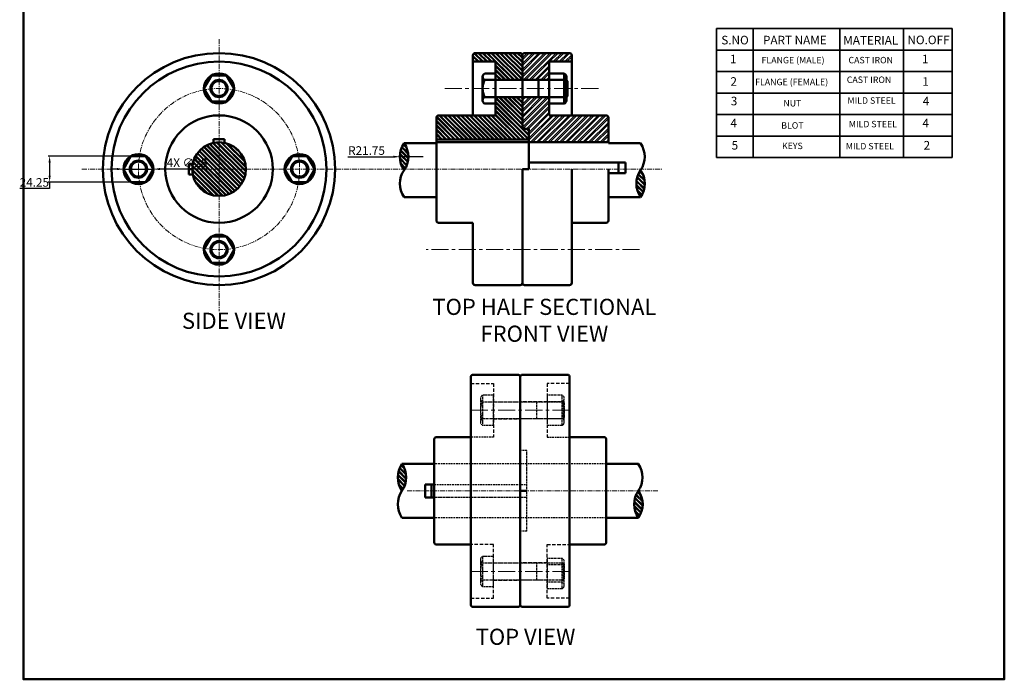
# Model space of a CAD drawing. Units: millimetres. Extents: x 36 to 952, y -590 to 448.
# Tile 1 of 2: x 36 to 952, y -590 to 24. Entities that reach past the tile are written whole.
import ezdxf

# ---------------------------------------------------------------- set-up
doc = ezdxf.new("R2010")
doc.units = ezdxf.units.MM
doc.header["$LTSCALE"] = 0.5
doc.linetypes.add('CENTER', pattern=[50.8, 31.75, -6.35, 6.35, -6.35])
doc.linetypes.add('HIDDEN', pattern=[9.525, 6.35, -3.175])
for name, color, linetype, lineweight in [('M-CNTR', 1, 'CENTER', 18), ('M-DIMS', 2, 'Continuous', 25), ('M-HATC', 8, 'Continuous', 18), ('M-HIDN', 4, 'HIDDEN', 25), ('M-OUTL', 7, 'Continuous', 50), ('M-TEXT', 7, 'Continuous', 25), ('M-TTLB', 7, 'Continuous', 35)]:
    doc.layers.add(name, color=color, linetype=linetype, lineweight=lineweight)
doc.styles.get("Standard").update_dxf_attribs({"font": 'arial.ttf'})
doc.dimstyles.new('ISO-25', dxfattribs={"dimtxt": 8, "dimasz": 6, "dimexe": 1.25, "dimexo": 0.625, "dimtad": 1, "dimtoh": 1, "dimtxsty": 'Standard', "dimcen": 2.5, "dimadec": 0, "dimazin": 0, "dimtfac": 1, "dimtmove": 0, "dimatfit": 3, "dimfxl": 1, "dimarcsym": 0})
pattern_1 = [(135, (903.4658, -449.5868), (-2.020558, -2.020558), []), (135, (903.4658, -448.2397), (-2.020558, -2.020558), [])]

# ---------------------------------------------------------------- blocks, each defined once
blk = doc.blocks.new('NUT-HEX')
at = {"ltscale": 0.3}
blk.add_lwpolyline([(28, 14), (21, 26.12), (7, 26.12), (0, 14), (7, 1.88), (21, 1.88)], close=True, dxfattribs=at)
blk.add_circle((14, 14), 14, dxfattribs=at)
blk = doc.blocks.new('*D27')
at = {"layer": 'Defpoints', "color": 0, "ltscale": 0.5, "transparency": 16777216}
for p in [(139.37, -102.71), (63.75, -126.96), (139.37, -126.96)]:
    blk.add_point(p, dxfattribs=at)
at = {"layer": 'M-DIMS', "color": 0, "lineweight": -2, "ltscale": 0.5, "transparency": 16777216}
for p, q in [((138.74, -102.71), (62.5, -102.71)), ((63.75, -108.71), (63.75, -120.96)), ((138.74, -126.96), (62.5, -126.96)), ((63.75, -126.96), (63.75, -132.96)), ((63.75, -132.96), (35.94, -132.96))]:
    blk.add_line(p, q, dxfattribs=at)
at = {"layer": 'M-DIMS', "color": 0, "ltscale": 0.5, "transparency": 16777216}
for points in [[(62.75, -108.71), (64.75, -108.71), (63.75, -102.71)], [(62.75, -120.96), (64.75, -120.96), (63.75, -126.96)]]:
    blk.add_solid(points, dxfattribs=at)
at = {"layer": 'M-DIMS', "color": 0, "ltscale": 0.5, "transparency": 16777216, "insert": (49.53, -128.25), "char_height": 8, "attachment_point": 5}
blk.add_mtext('24.25', dxfattribs=at)
blk = doc.blocks.new('*D30')
at = {"layer": 'Defpoints', "color": 0, "ltscale": 0.5, "transparency": 16777216}
for p in [(132.37, -114.83), (160.37, -114.83)]:
    blk.add_point(p, dxfattribs=at)
at = {"layer": 'M-DIMS', "color": 0, "lineweight": -2, "ltscale": 0.5, "transparency": 16777216}
for p, q in [((126.37, -114.83), (120.37, -114.83)), ((132.37, -114.83), (160.37, -114.83)), ((172.37, -114.83), (166.37, -114.83)), ((210.26, -114.83), (172.37, -114.83))]:
    blk.add_line(p, q, dxfattribs=at)
at = {"layer": 'M-DIMS', "color": 0, "ltscale": 0.5, "transparency": 16777216}
for points in [[(126.37, -113.83), (126.37, -115.83), (132.37, -114.83)], [(166.37, -113.83), (166.37, -115.83), (160.37, -114.83)]]:
    blk.add_solid(points, dxfattribs=at)
at = {"layer": 'M-DIMS', "color": 0, "ltscale": 0.5, "transparency": 16777216, "insert": (191.62, -109.9), "char_height": 8, "attachment_point": 5}
blk.add_mtext('4X ∅28', dxfattribs=at)
blk = doc.blocks.new('*D31')
at = {"layer": 'Defpoints', "color": 0, "ltscale": 0.5, "transparency": 16777216}
for p in [(389.66, -103.33), (411.41, -103.33)]:
    blk.add_point(p, dxfattribs=at)
at = {"layer": 'M-DIMS', "color": 0, "lineweight": -2, "ltscale": 0.5, "transparency": 16777216}
for p, q in [((341.28, -103.33), (376.61, -103.33)), ((376.61, -103.33), (383.66, -103.33)), ((411.41, -103.33), (389.66, -103.33))]:
    blk.add_line(p, q, dxfattribs=at)
at = {"layer": 'M-DIMS', "color": 0, "ltscale": 0.5, "transparency": 16777216}
blk.add_solid([(383.66, -102.33), (383.66, -104.33), (389.66, -103.33)], dxfattribs=at)
at = {"layer": 'M-DIMS', "color": 0, "ltscale": 0.5, "transparency": 16777216, "insert": (358.63, -98.62), "char_height": 8, "attachment_point": 5}
blk.add_mtext('R21.75', dxfattribs=at)

msp = doc.modelspace()

# ---------------------------------------------------------------- hatches: boundary and pattern name
at = {"layer": 'M-HATC', "ltscale": 0.3}
h = msp.add_hatch(dxfattribs=at)
h.set_pattern_fill('ANSI32', color=256, scale=0.3, angle=90)
h.set_pattern_definition([(135, (649.1825, -488.8874), (-2.020558, -2.020558), []), (135, (649.1825, -487.5403), (-2.020558, -2.020558), [])])
h.paths.add_polyline_path([(459.614, -6.832, 0.4142136), (457.614, -8.832), (457.614, -14.832), (478.614, -14.832), (478.614, -31.832), (503.614, -31.832), (503.614, -8.832, 0.4142136), (501.614, -6.832)])
h = msp.add_hatch(dxfattribs=at)
h.set_pattern_fill('ANSI32', color=256, scale=0.4)
h.set_pattern_definition([(45, (47.152, -333.0392), (-2.694077, 2.694077), []), (45, (48.948, -333.0392), (-2.694077, 2.694077), [])])
h.paths.add_polyline_path([(528.614, -14.832), (549.614, -14.832), (549.614, -8.832, 0.4142136), (547.614, -6.832), (505.614, -6.832, 0.4142136), (503.614, -8.832), (503.614, -31.832), (528.614, -31.832)])
h.paths.add_polyline_path([(503.614, -77.332), (509.614, -77.332), (509.614, -89.832), (583.614, -89.832), (583.614, -66.832, 0.4142136), (581.614, -64.832), (528.614, -64.832), (528.614, -47.832), (503.614, -47.832)])
h = msp.add_hatch(dxfattribs=at)
h.set_pattern_fill('ANSI32', color=256, scale=0.3, angle=90)
h.set_pattern_definition(pattern_1)
h.paths.add_polyline_path([(478.614, -64.832), (425.614, -64.832, 0.4142136), (423.614, -66.832), (423.614, -87.332), (509.614, -87.332), (509.614, -77.332), (503.614, -77.332), (503.614, -47.832), (478.614, -47.832)])
h = msp.add_hatch(dxfattribs=at)
h.set_pattern_fill('ANSI32', color=256, scale=0.3, angle=90)
h.set_pattern_definition([(135, (1009.3846, -92.6427), (-2.020558, -2.020558), []), (135, (1009.3846, -91.2956), (-2.020558, -2.020558), [])])
h.paths.add_polyline_path([(196.366, -114.832), (246.366, -114.832, 1)])
h.paths.add_polyline_path([(246.366, -114.832), (196.366, -114.832, 1)])
h = msp.add_hatch(dxfattribs=at)
h.set_pattern_fill('ANSI32', color=256, scale=0.3, angle=90)
h.set_pattern_definition(pattern_1)
h.paths.add_polyline_path([(393.614, -115.832, 0.31606), (393.614, -90.832, 0.31606)])
h = msp.add_hatch(dxfattribs=at)
h.set_pattern_fill('ANSI32', color=256, scale=0.3, angle=90)
h.set_pattern_definition([(135, (1123.4658, -474.5868), (-2.020558, -2.020558), []), (135, (1123.4658, -473.2397), (-2.020558, -2.020558), [])])
h.paths.add_polyline_path([(613.614, -140.832, 0.31606), (613.614, -115.832, 0.31606)])
h = msp.add_hatch(dxfattribs=at)
h.set_pattern_fill('ANSI32', color=256, scale=0.3, angle=90)
h.set_pattern_definition([(135, (901.4658, -748.1027), (-2.020558, -2.020558), []), (135, (901.4658, -746.7557), (-2.020558, -2.020558), [])])
h.paths.add_polyline_path([(391.614, -414.348, 0.31606), (391.614, -389.348, 0.31606)])
h = msp.add_hatch(dxfattribs=at)
h.set_pattern_fill('ANSI32', color=256, scale=0.3, angle=90)
h.set_pattern_definition([(135, (1121.4658, -773.1027), (-2.020558, -2.020558), []), (135, (1121.4658, -771.7557), (-2.020558, -2.020558), [])])
h.paths.add_polyline_path([(611.614, -439.348, 0.31606), (611.614, -414.348, 0.31606)])

# ---------------------------------------------------------------- linework, layer by layer
at = {"layer": 'M-CNTR', "ltscale": 0.3}
for p, q in [((221.366, 6.13), (221.366, -247.228)), ((93.755, -114.832), (633.407, -114.832)), ((396.436, -414.348), (629.872, -414.348))]:
    msp.add_line(p, q, dxfattribs=at)
at = {"layer": 'M-CNTR'}
for p, q in [((574.352, -39.832), (431.256, -39.832)), ((612.663, -189.832), (414.062, -189.832)), ((455.614, -339.348), (501.614, -339.348)), ((547.614, -339.348), (501.614, -339.348)), ((455.614, -489.348), (501.614, -489.348)), ((547.614, -489.348), (501.614, -489.348))]:
    msp.add_line(p, q, dxfattribs=at)
at = {"layer": 'M-CNTR', "ltscale": 0.3}
msp.add_circle((221.366, -114.832), 75, dxfattribs=at)
at = {"layer": 'M-HIDN'}
for p, q in [((455.614, -314.348), (476.614, -314.348)), ((476.614, -314.348), (476.614, -364.348)), ((547.614, -314.348), (526.614, -314.348)), ((526.614, -314.348), (526.614, -364.348)), ((476.614, -331.348), (501.614, -331.348)), ((526.614, -331.348), (501.614, -331.348)), ((476.614, -347.348), (501.614, -347.348)), ((526.614, -347.348), (501.614, -347.348)), ((476.614, -464.348), (455.614, -464.348)), ((476.614, -514.348), (476.614, -464.348)), ((526.614, -514.348), (526.614, -464.348)), ((526.614, -464.348), (547.614, -464.348)), ((476.614, -481.348), (501.614, -481.348)), ((526.614, -481.348), (501.614, -481.348)), ((476.614, -497.348), (501.614, -497.348)), ((526.614, -497.348), (501.614, -497.348)), ((455.614, -514.348), (476.614, -514.348)), ((547.614, -514.348), (526.614, -514.348))]:
    msp.add_line(p, q, dxfattribs=at)
at = {"layer": 'M-HIDN', "ltscale": 0.3}
for p, q in [((464.614, -328.348), (464.614, -347.348)), ((476.614, -325.348), (466.614, -325.348)), ((466.614, -325.348), (466.614, -353.348)), ((476.614, -331.348), (476.614, -325.348)), ((540.614, -325.348), (526.614, -325.348)), ((526.614, -325.348), (526.614, -353.348)), ((540.614, -353.348), (540.614, -325.348)), ((542.614, -350.348), (542.614, -328.348)), ((464.614, -331.348), (541.614, -331.348)), ((476.614, -347.348), (476.614, -331.348)), ((516.614, -331.348), (516.614, -347.348)), ((540.614, -331.348), (526.614, -331.348)), ((542.614, -332.348), (541.614, -331.348)), ((541.614, -331.348), (541.614, -347.348)), ((542.614, -332.348), (542.614, -346.348)), ((541.614, -347.348), (464.614, -347.348)), ((464.614, -347.348), (464.614, -350.348)), ((476.614, -353.348), (476.614, -347.348)), ((540.614, -347.348), (526.614, -347.348)), ((542.614, -346.348), (541.614, -347.348)), ((466.614, -353.348), (476.614, -353.348)), ((526.614, -353.348), (540.614, -353.348)), ((507.614, -420.598), (421.614, -420.598)), ((476.614, -475.348), (466.614, -475.348)), ((466.614, -475.348), (466.614, -503.348)), ((476.614, -481.348), (476.614, -475.348)), ((464.614, -478.348), (464.614, -497.348)), ((464.614, -481.348), (541.614, -481.348)), ((476.614, -497.348), (476.614, -481.348)), ((516.614, -481.348), (516.614, -497.348)), ((540.614, -477.348), (526.614, -477.348)), ((526.614, -477.348), (526.614, -505.348)), ((540.614, -483.348), (526.614, -483.348)), ((540.614, -505.348), (540.614, -477.348)), ((542.614, -482.348), (541.614, -481.348)), ((541.614, -481.348), (541.614, -497.348)), ((542.614, -502.348), (542.614, -480.348)), ((542.614, -482.348), (542.614, -496.348)), ((541.614, -497.348), (464.614, -497.348)), ((464.614, -497.348), (464.614, -500.348)), ((466.614, -503.348), (476.614, -503.348)), ((476.614, -503.348), (476.614, -497.348)), ((540.614, -499.348), (526.614, -499.348)), ((542.614, -496.348), (541.614, -497.348)), ((526.614, -505.348), (540.614, -505.348))]:
    msp.add_line(p, q, dxfattribs=at)
at = {"layer": 'M-HIDN', "ltscale": 0.5}
for p, q in [((476.614, -364.348), (455.614, -364.348)), ((526.614, -364.348), (547.614, -364.348)), ((507.614, -376.848), (501.614, -376.848)), ((581.614, -389.348), (421.614, -389.348)), ((421.614, -408.598), (507.614, -408.598)), ((581.614, -439.348), (421.614, -439.348)), ((507.614, -451.848), (501.614, -451.848))]:
    msp.add_line(p, q, dxfattribs=at)
at = {"layer": 'M-HIDN', "ltscale": 0.3}
msp.add_lwpolyline([(507.614, -451.848), (507.614, -414.348), (507.614, -376.848)], dxfattribs=at)
for centre, radius, start, end in [((467.864, -328.348), 3.25, 112.619865, 247.380135), ((539.364, -328.348), 3.25, 292.619865, 67.380135), ((481.614, -339.348), 17, 151.927513, 208.072487), ((525.614, -339.348), 17, 331.927513, 28.072487), ((467.864, -350.348), 3.25, 112.619865, 247.380135), ((539.364, -350.348), 3.25, 292.619865, 67.380135), ((467.864, -478.348), 3.25, 112.619865, 247.380135), ((481.614, -489.348), 17, 151.927513, 208.072487), ((539.364, -480.348), 3.25, 292.619865, 67.380135), ((525.614, -491.348), 17, 331.927513, 28.072487), ((467.864, -500.348), 3.25, 112.619865, 247.380135), ((539.364, -502.348), 3.25, 292.619865, 67.380135)]:
    msp.add_arc(centre, radius, start, end, dxfattribs=at)
at = {"layer": 'M-OUTL'}
for p, q in [((457.614, -8.832), (457.614, -64.832)), ((459.614, -6.832), (501.614, -6.832)), ((503.614, -8.832), (503.614, -77.332)), ((503.614, -8.832), (503.614, -77.332)), ((505.614, -6.832), (547.614, -6.832)), ((549.614, -8.832), (549.614, -64.832)), ((457.614, -14.832), (478.614, -14.832)), ((478.614, -14.832), (478.614, -64.832)), ((549.614, -14.832), (528.614, -14.832)), ((528.614, -14.832), (528.614, -64.832)), ((478.614, -31.832), (503.614, -31.832)), ((528.614, -31.832), (503.614, -31.832)), ((478.614, -47.832), (503.614, -47.832)), ((528.614, -47.832), (503.614, -47.832)), ((423.614, -66.832), (423.614, -114.832)), ((478.614, -64.832), (425.614, -64.832)), ((528.614, -64.832), (581.614, -64.832)), ((583.614, -66.832), (583.614, -90.832)), ((503.614, -77.332), (508.614, -77.332)), ((509.614, -87.332), (423.614, -87.332)), ((509.614, -89.832), (423.614, -89.832)), ((509.614, -89.832), (583.614, -89.832)), ((423.614, -162.832), (423.614, -114.832)), ((549.614, -220.832), (549.614, -114.832)), ((583.614, -162.832), (583.614, -114.832)), ((503.614, -135.203), (503.614, -139.832)), ((503.614, -220.832), (503.614, -152.332)), ((503.614, -220.832), (503.614, -152.332)), ((457.614, -220.832), (457.614, -164.832)), ((459.614, -222.832), (501.614, -222.832)), ((505.614, -222.832), (547.614, -222.832)), ((455.614, -308.348), (455.614, -464.348)), ((457.614, -306.348), (499.614, -306.348)), ((501.614, -308.348), (501.614, -376.848)), ((501.614, -308.348), (501.614, -420.598)), ((503.614, -306.348), (545.614, -306.348)), ((547.614, -308.348), (547.614, -420.598)), ((421.614, -366.348), (421.614, -414.348)), ((455.614, -364.348), (423.614, -364.348)), ((547.614, -364.348), (579.614, -364.348)), ((581.614, -366.348), (581.614, -414.348)), ((421.614, -462.348), (421.614, -414.348)), ((547.614, -520.348), (547.614, -420.598)), ((581.614, -462.348), (581.614, -414.348)), ((501.614, -434.719), (501.614, -439.348)), ((501.614, -520.348), (501.614, -451.848)), ((501.614, -520.348), (501.614, -451.848)), ((455.614, -520.348), (455.614, -464.348)), ((457.614, -522.348), (499.614, -522.348)), ((503.614, -522.348), (545.614, -522.348))]:
    msp.add_line(p, q, dxfattribs=at)
at = {"layer": 'M-OUTL', "ltscale": 0.3}
for p, q in [((478.614, -25.832), (468.614, -25.832)), ((478.614, -31.832), (478.614, -25.832)), ((542.614, -25.832), (528.614, -25.832)), ((528.614, -25.832), (528.614, -53.832)), ((542.614, -53.832), (542.614, -25.832)), ((466.614, -28.832), (466.614, -47.832)), ((466.614, -31.832), (543.614, -31.832)), ((478.614, -53.832), (478.614, -31.832)), ((518.614, -31.832), (518.614, -47.832)), ((544.614, -31.832), (528.614, -31.832)), ((544.614, -50.832), (544.614, -28.832)), ((545.614, -32.832), (544.614, -31.832)), ((544.614, -31.832), (544.614, -47.832)), ((544.614, -32.832), (544.614, -46.832)), ((545.614, -46.832), (545.614, -32.832)), ((543.614, -47.832), (466.614, -47.832)), ((466.614, -47.832), (466.614, -50.832)), ((468.614, -53.832), (478.614, -53.832)), ((544.614, -47.832), (528.614, -47.832)), ((528.614, -53.832), (542.614, -53.832)), ((545.614, -46.832), (544.614, -47.832)), ((503.614, -77.332), (509.614, -77.332)), ((509.614, -77.332), (509.614, -114.832)), ((221.366, -86.832), (216.366, -86.832)), ((216.366, -86.832), (216.366, -90.337)), ((221.366, -86.832), (226.366, -86.832)), ((226.366, -86.832), (226.366, -90.337)), ((423.614, -90.832), (393.614, -90.832)), ((583.614, -90.832), (613.614, -90.832)), ((193.366, -114.832), (193.366, -109.832)), ((193.366, -109.832), (196.871, -109.832)), ((509.614, -108.582), (599.614, -108.582)), ((593.028, -108.582), (593.028, -118.582)), ((599.614, -108.582), (599.614, -118.582)), ((196.366, -114.832), (193.366, -114.832)), ((193.366, -114.832), (193.366, -119.832)), ((503.614, -152.332), (503.614, -114.832)), ((509.614, -114.832), (503.614, -114.832)), ((599.614, -118.582), (583.614, -118.582)), ((193.366, -119.832), (196.871, -119.832)), ((503.614, -152.332), (503.614, -135.203)), ((393.614, -140.832), (423.614, -140.832)), ((613.614, -140.832), (583.614, -140.832)), ((425.614, -164.832), (457.614, -164.832)), ((581.614, -164.832), (549.614, -164.832)), ((421.614, -389.348), (391.614, -389.348)), ((501.614, -420.598), (501.614, -386.848)), ((581.614, -389.348), (611.614, -389.348)), ((501.614, -420.598), (501.614, -414.348)), ((507.614, -414.348), (501.614, -414.348)), ((501.614, -451.848), (501.614, -420.598)), ((391.614, -439.348), (421.614, -439.348)), ((501.614, -451.848), (501.614, -434.719)), ((611.614, -439.348), (581.614, -439.348)), ((423.614, -464.348), (455.614, -464.348)), ((579.614, -464.348), (547.614, -464.348))]:
    msp.add_line(p, q, dxfattribs=at)
at = {"layer": 'M-OUTL', "ltscale": 0.5}
for p, q in [((413.123, -420.598), (413.123, -408.598)), ((413.123, -408.598), (421.614, -408.598)), ((419.19, -408.598), (419.19, -420.598)), ((421.614, -420.598), (413.123, -420.598))]:
    msp.add_line(p, q, dxfattribs=at)
msp.add_lwpolyline([(39.441, 448.041), (952.031, 448.041), (952.031, -589.796), (39.441, -589.796)], close=True, dxfattribs=at)
at = {"layer": 'M-OUTL', "ltscale": 0.3}
for centre, radius in [((221.366, -114.832), 108), ((221.366, -114.832), 100), ((221.366, -39.832), 8), ((221.366, -39.832), 7), ((221.366, -114.832), 50), ((221.366, -114.832), 25), ((146.366, -114.832), 8), ((146.366, -114.832), 7), ((296.366, -114.832), 8), ((296.366, -114.832), 7), ((221.366, -189.832), 8), ((221.366, -189.832), 7)]:
    msp.add_circle(centre, radius, dxfattribs=at)
at = {"layer": 'M-OUTL'}
for centre, start, end in [((459.614, -8.832), 90, 180), ((501.614, -8.832), 0, 90), ((505.614, -8.832), 90, 180), ((547.614, -8.832), 0, 90), ((425.614, -66.832), 90, 180), ((581.614, -66.832), 0, 90), ((459.614, -220.832), 180, 270), ((501.614, -220.832), 270, 0), ((505.614, -220.832), 180, 270), ((547.614, -220.832), 270, 0), ((457.614, -308.348), 90, 180), ((499.614, -308.348), 0, 90), ((503.614, -308.348), 90, 180), ((545.614, -308.348), 0, 90), ((423.614, -366.348), 90, 180), ((579.614, -366.348), 0, 90), ((457.614, -520.348), 180, 270), ((499.614, -520.348), 270, 0), ((503.614, -520.348), 180, 270), ((545.614, -520.348), 270, 0)]:
    msp.add_arc(centre, 2, start, end, dxfattribs=at)
at = {"layer": 'M-OUTL', "ltscale": 0.3}
for centre, radius, start, end in [((469.864, -28.832), 3.25, 112.619865, 247.380135), ((541.364, -28.832), 3.25, 292.619865, 67.380135), ((483.614, -39.832), 17, 151.927513, 208.072487), ((527.614, -39.832), 17, 331.927513, 28.072487), ((469.864, -50.832), 3.25, 112.619865, 247.380135), ((541.364, -50.832), 3.25, 292.619865, 67.380135), ((411.413, -103.332), 21.75, 144.920681, 215.079319), ((375.814, -103.332), 21.75, 324.920681, 35.079319), ((595.707, -103.332), 21.75, 324.920681, 35.079319), ((411.413, -128.332), 21.75, 144.920681, 215.079319), ((631.413, -128.332), 21.75, 144.920681, 215.079319), ((595.814, -128.332), 21.75, 324.920681, 35.079319), ((425.614, -162.832), 2, 180, 270), ((581.614, -162.832), 2, 270, 0), ((409.413, -401.848), 21.75, 144.920681, 215.079319), ((373.814, -401.848), 21.75, 324.920681, 35.079319), ((593.707, -401.848), 21.75, 324.920681, 35.079319), ((409.413, -426.848), 21.75, 144.920681, 215.079319), ((629.413, -426.848), 21.75, 144.920681, 215.079319), ((593.814, -426.848), 21.75, 324.920681, 35.079319), ((423.614, -462.348), 2, 180, 270), ((579.614, -462.348), 2, 270, 0)]:
    msp.add_arc(centre, radius, start, end, dxfattribs=at)
at = {"layer": 'M-TTLB', "ltscale": 0.5}
for p, q in [((684.39, 15.948), (903.629, 15.948)), ((684.39, -104.052), (684.39, 15.948)), ((718.214, 15.948), (718.214, -104.052)), ((799.009, 15.955), (799.009, -104.045)), ((858.232, 15.948), (858.232, -104.052)), ((903.629, 15.948), (903.629, -104.052)), ((684.39, -4.052), (903.629, -4.052)), ((684.39, -24.052), (903.629, -24.052)), ((684.39, -44.052), (903.629, -44.052)), ((684.39, -64.052), (903.629, -64.052)), ((684.39, -84.052), (903.629, -84.052)), ((903.629, -104.052), (684.39, -104.052))]:
    msp.add_line(p, q, dxfattribs=at)

# ---------------------------------------------------------------- block references
at = {"layer": 'M-OUTL'}
for p in [(207.366, -53.832), (132.366, -128.832), (282.366, -128.832), (207.366, -203.832)]:
    msp.add_blockref('NUT-HEX', p, dxfattribs=at)

# ---------------------------------------------------------------- texts
at = {"layer": 'M-TEXT', "ltscale": 0.5, "attachment_point": 1}
for s, width, insert, char_height in [('\\pxqc;S.NO', 16.26852, (693.34, 9.249), 8), ('\\pxqc;PART NAME', 68.15745, (723.056, 9.249), 8), ('\\pxqc;NO.OFF', 16.26852, (873.345, 9.415), 8), ('\\pxqc;MATERIAL', 68.15745, (793.696, 9.083), 8), ('\\pxqc;1', 15.29946, (692.205, -8.412), 8), ('\\pxqc;1', 15.29946, (870.819, -8.412), 8), ('\\pxqc;FLANGE (MALE)', 63.57663, (723.697, -10.377), 6), ('\\pxqc;CAST IRON', 50.31101, (802.57, -10.377), 6), ('\\pxqc;2', 9.45073, (695.519, -29.291), 8), ('\\pxql;FLANGE (FEMALE)', 76.03571, (720.214, -30.746), 6), ('\\pxqc;CAST IRON', 47.80909, (802.258, -28.652), 6), ('\\pxqc;1', 9.45073, (874.133, -29.291), 8), ('\\pxqc;3', 12.88084, (694.148, -47.469), 8), ('\\pxqc;NUT', 50.31101, (729.704, -50.557), 6), ('\\pxqc;MILD STEEL', 48.84582, (804.125, -48.016), 6), ('\\pxqc;4', 12.88084, (872.762, -47.469), 8), ('\\pxqc;4', 12.03604, (694.243, -67.979), 8), ('\\pxqc;BLOT', 50.31101, (729.704, -71.208), 6), ('\\pxqc;MILD STEEL', 48.84582, (805.354, -69.934), 6), ('\\pxqc;4', 12.03604, (872.857, -67.979), 8), ('\\pxqc;5', 13.25303, (694.72, -88.648), 8), ('\\pxqc;KEYS', 50.31101, (729.704, -90.232), 6), ('\\pxqc;MILD STEEL', 48.84582, (802.56, -90.506), 6), ('\\pxqc;2', 13.25303, (873.333, -88.648), 8)]:
    msp.add_mtext_dynamic_manual_height_columns(s, width=width, gutter_width=12.5, heights=[0], dxfattribs=dict(at, insert=insert, char_height=char_height))
at = {"layer": 'M-TEXT', "ltscale": 0.3, "char_height": 15, "attachment_point": 1}
for s, width, insert in [('\\pxqc;TOP HALF SECTIONAL FRONT VIEW', 278.15027, (385.01, -235.579)), ('\\pxqc;SIDE VIEW', 148.39271, (161.028, -248.553)), ('\\pxqc;TOP VIEW', 189.76886, (411.686, -542.697))]:
    msp.add_mtext_dynamic_manual_height_columns(s, width=width, gutter_width=12.5, heights=[0], dxfattribs=dict(at, insert=insert))

# ---------------------------------------------------------------- dimensions: what is measured, and where the dimension line sits
at = {"layer": 'M-DIMS', "ltscale": 0.5}
dim = msp.add_diameter_dim_2p(p1=(132.366, -114.832), p2=(160.366, -114.832), text='4X <>', dimstyle='ISO-25', override={"dimdec": 0, "dimlfac": 1, "dimrnd": 0, "dimzin": 0, "dimdsep": 46, "dimlunit": 2}, dxfattribs=at)
dim.commit()
dim.dimension.update_dxf_attribs({"geometry": '*D30', "text_midpoint": (172.366, -114.832), "dimtype": 163})
dim = msp.add_radius_dim(center=(411.413, -103.332), mpoint=(389.663, -103.332), dimstyle='ISO-25', override={"dimdec": 2, "dimlfac": 1, "dimrnd": 0, "dimzin": 0, "dimdsep": 46, "dimlunit": 2}, dxfattribs=at)
dim.commit()
dim.dimension.update_dxf_attribs({"geometry": '*D31', "text_midpoint": (376.613, -103.332), "dimtype": 164})
dim = msp.add_linear_dim(base=(63.755, -126.957), p1=(139.366, -102.708), p2=(139.366, -126.957), angle=90, dimstyle='ISO-25', override={"dimdec": 2, "dimlfac": 1, "dimrnd": 0, "dimzin": 0, "dimdsep": 46, "dimlunit": 2}, dxfattribs=at)
dim.commit()
dim.dimension.update_dxf_attribs({"geometry": '*D27', "text_midpoint": (49.534, -128.247)})

doc.saveas('drawing.dxf')
